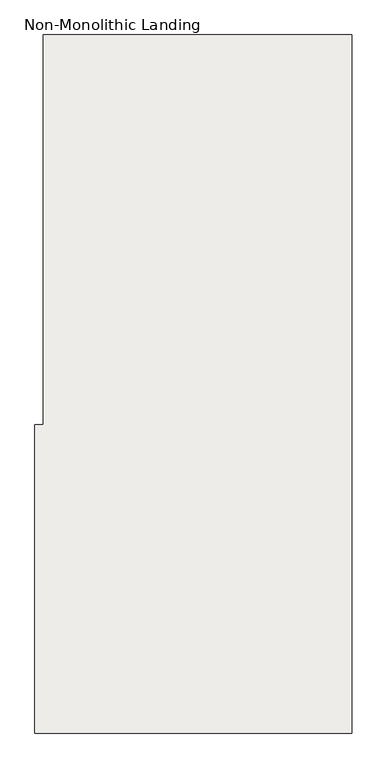
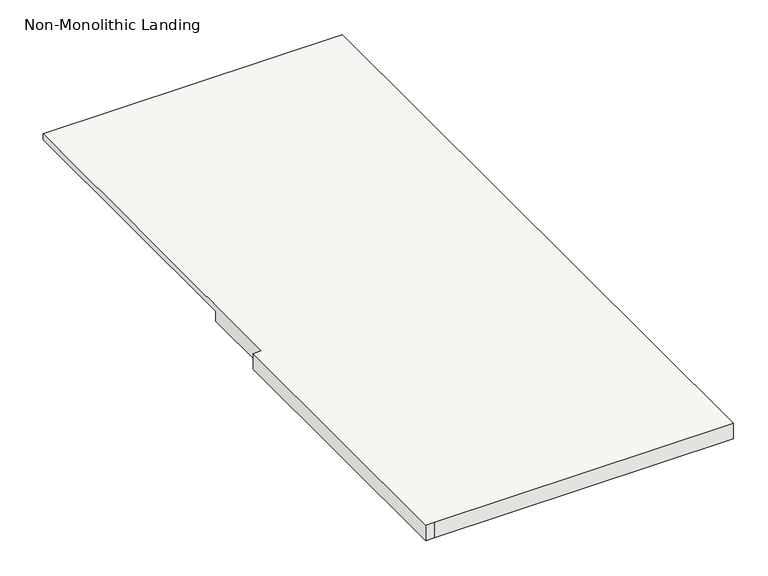
"""IFC4 building model written with IfcOpenShell, lengths in millimetres: slab geometry, Non-Monolithic Landing."""

from ifc_helpers import new_model, si_unit, origin, place, context, project, spatial, faceted_brep, source, transform, mapped, element, save


def non_monolithic_landing_9c4d403a(model_context):
    return source(origin(), model_context, "Body", "Brep", [
        faceted_brep([(-2178.613859, 1358.5428136, 1581.15), (-2153.213859, 1358.5428136, 1555.75), (-2153.213859, 444.1428136, 1555.75), (-2178.613859, 444.1428136, 1581.15), (-2178.613859, 202.2206867, 1600.2), (-2204.013859, 202.2206867, 1600.2), (-2204.013859, -712.1793133, 1600.2), (-2178.613859, -712.1793133, 1600.2), (-1264.213859, -712.1793133, 1600.2), (-1264.213859, 1358.5428136, 1600.2), (-2178.613859, 1358.5428136, 1600.2), (-2153.213859, 444.1428136, 1549.4), (-2153.213859, 1358.5428136, 1549.4), (-1264.213859, 1358.5428136, 1549.4), (-1264.213859, -712.1793133, 1549.4), (-2178.613859, -712.1793133, 1549.4), (-2204.013859, -712.1793133, 1549.4), (-2204.013859, 202.2206867, 1549.4), (-2178.613859, 202.2206867, 1549.4), (-2178.613859, 444.1428136, 1549.4)], [[[0, 1, 2, 3]], [[4, 5, 6, 7, 8, 9, 10]], [[11, 12, 13, 14, 15, 16, 17, 18, 19]], [[12, 11, 2, 1]], [[11, 19, 3, 2]], [[4, 10, 0, 3, 19, 18]], [[5, 4, 18, 17]], [[6, 5, 17, 16]], [[7, 6, 16, 15]], [[8, 7, 15, 14]], [[9, 8, 14, 13]], [[10, 9, 13, 12, 1, 0]]]),
    ])


if __name__ == "__main__":
    model = new_model("IFC4")
    model_context = context("Model", 3, world=origin())
    ifc_project = project(units=[si_unit("LENGTHUNIT", "METRE", prefix="MILLI")], contexts=[model_context])
    site = spatial("IfcSite", under=ifc_project)
    building = spatial("IfcBuilding", under=site)
    placement = place(None, origin())
    non_monolithic_landing_shape = non_monolithic_landing_9c4d403a(model_context)
    element("IfcSlab", 1, ObjectType="Non-Monolithic Landing", at=placement, inside=building, context=model_context, shape_type="MappedRepresentation", body=[
        mapped(non_monolithic_landing_shape, transform((0.0, 0.0, 0.0), x_axis=(1.0, 0.0, 0.0), y_axis=(0.0, 1.0, 0.0), z_axis=(0.0, 0.0, 1.0))),
    ])
    save(model, "model.ifc")
